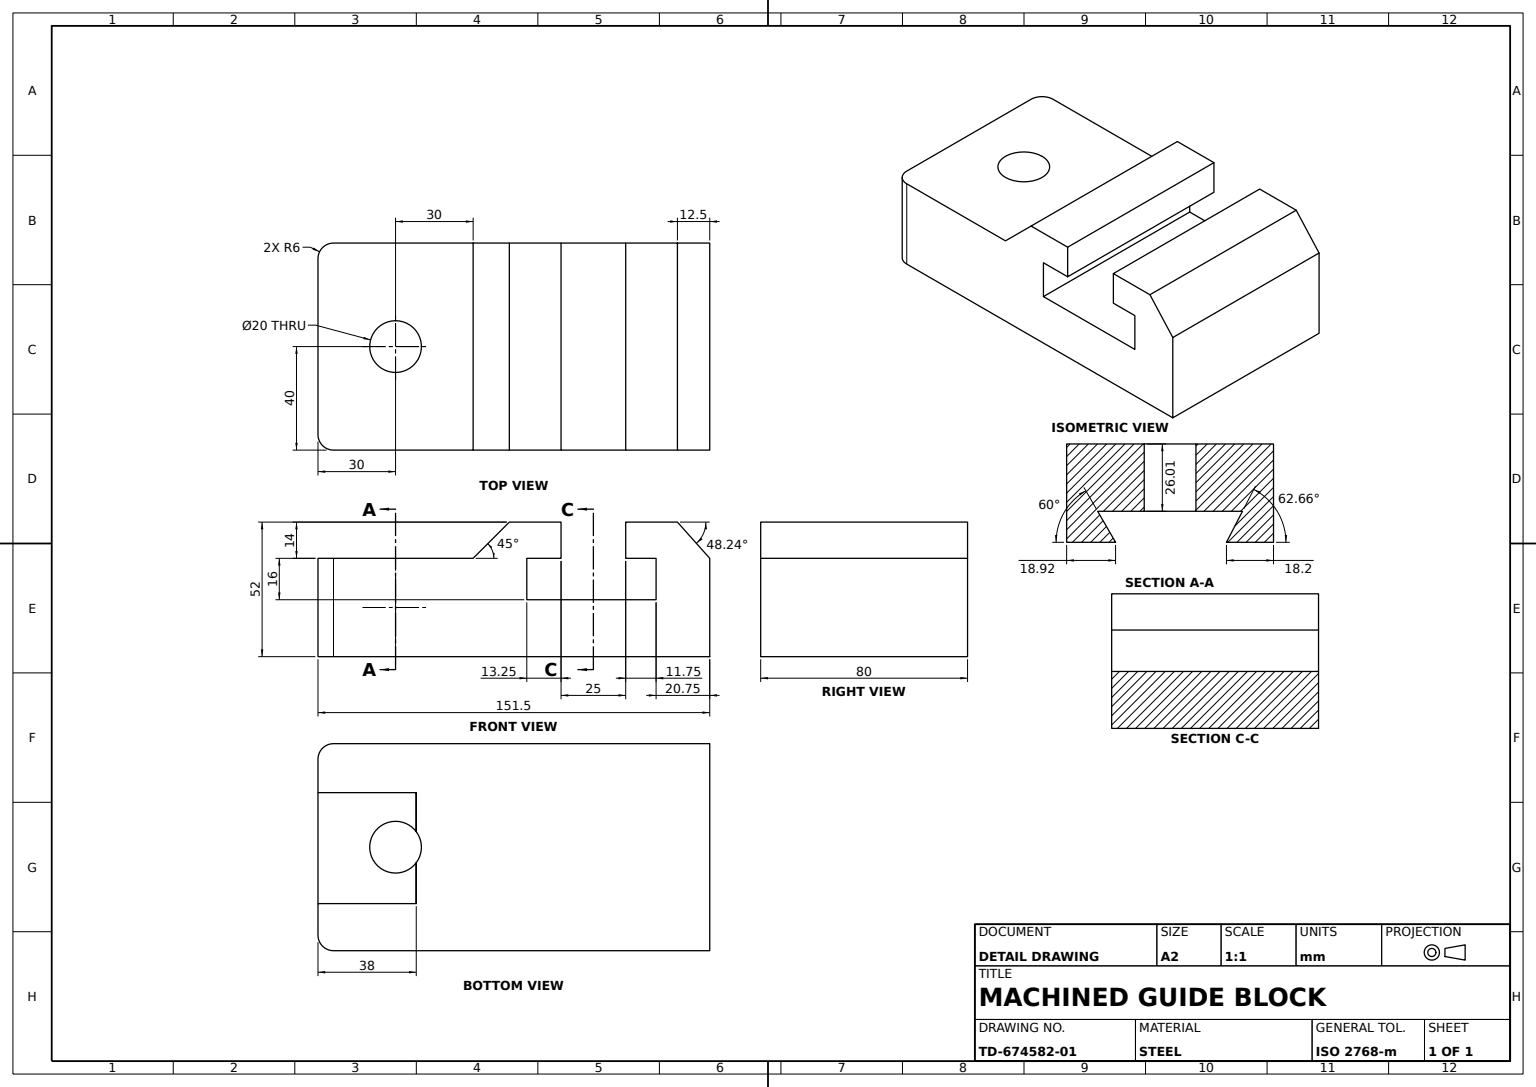
from build123d import *

# Parameters (mm, degrees)
BASE_BODY_DEPTH    = 80
RAISED_BLOCK_DEPTH = 38
WEDGE_BOSS_DEPTH   = 80
TOP_HOLE_SKETCH_R  = 10
TOP_HOLE_DEPTH     = 38
PROFILE_CUT_DEPTH  = 38


with BuildPart() as part:
    # Base Profile Sketch → Base Body (new body)
    with BuildSketch(Plane.XY):
        with BuildLine():
            Line((52.5, 0), (54, 0))
            Line((54, 0), (144, 0))
            Line((144, 0), (144, 22))
            Line((144, 22), (144, 38))
            Line((144, 38), (131.5, 52))
            Line((131.5, 52), (111.5, 52))
            Line((111.5, 52), (111.5, 38))
            Line((111.5, 38), (123.25, 38))
            Line((123.25, 38), (123.25, 22))
            Line((123.25, 22), (73.25, 22))
            Line((73.25, 22), (73.25, 38))
            Line((73.25, 38), (86.5, 38))
            Line((86.5, 38), (86.5, 52))
            Line((86.5, 52), (66.5, 52))
            Line((66.5, 52), (52.5, 38))
            Line((52.5, 38), (-1.5, 38))
            Line((-1.5, 38), (-1.5, 0))
            ThreePointArc((-1.5, 0), (-0.743974245, 0.047821822), (0, 0.190524981))
            Line((0, 0.190524981), (0, 0))
            Line((0, 0), (52.5, 0))
        make_face()
    extrude(amount=BASE_BODY_DEPTH)

    # Raised Block Sketch → Raised Block (add)
    with BuildSketch(Plane(origin=(0, 38, 0), x_dir=(1, 0, 0), z_dir=(0, 1, 0))):
        with BuildLine():
            Line((-1.5, 0), (-1.5, -6))
            Line((-1.5, -6), (-1.5, -74))
            Line((-1.5, -74), (-1.5, -80))
            ThreePointArc((-1.5, -80), (-5.742640687, -78.242640687), (-7.5, -74))
            Line((-7.5, -74), (-7.5, -6))
            ThreePointArc((-7.5, -6), (-5.742640687, -1.757359313), (-1.5, 0))
        make_face()
    extrude(amount=-RAISED_BLOCK_DEPTH)

    # Wedge Sketch → Wedge Boss (add)
    with BuildSketch(Plane(origin=(0, 0, 0), x_dir=(-1, 0, 0), z_dir=(0, 0, -1))):
        Polygon((0, 0.190524981), (0, 0), (1.5, 0), align=None)
    extrude(amount=-WEDGE_BOSS_DEPTH)

    # Top Hole Sketch → Top Hole (cut)
    with BuildSketch(Plane(origin=(0, 38, 0), x_dir=(1, 0, 0), z_dir=(0, 1, 0))):
        with Locations(Location((22.5, -40, 0), (0, 0, 270))):
            Circle(TOP_HOLE_SKETCH_R)
    extrude(amount=-TOP_HOLE_DEPTH, mode=Mode.SUBTRACT)

    # Profile Cut Sketch → Profile Cut (cut)
    with BuildSketch(Plane.ZY.offset(7.5)):
        Polygon((68, 11.989734921), (40, 11.989734921), (12, 11.989734921), (18.2, 0), (40, 0), (61.077723316, 0), align=None)
    extrude(amount=-PROFILE_CUT_DEPTH, mode=Mode.SUBTRACT)


solid = part.part
